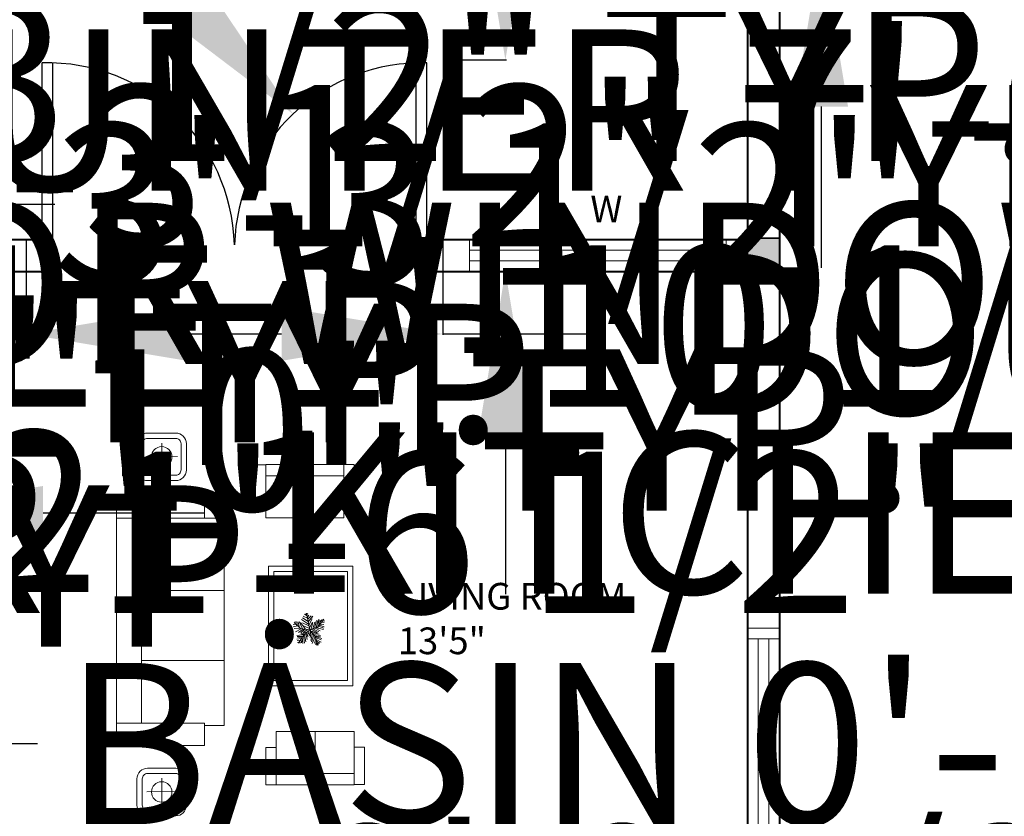
# Model space of a CAD drawing. Units: inches. Extents: x 7323 to 9737, y 2037 to 3322.
# Tile 14 of 19: x 9130 to 9314, y 2411 to 2560. Entities that reach past the tile are written whole.
import ezdxf

# ---------------------------------------------------------------- set-up
doc = ezdxf.new("R2010")
doc.units = ezdxf.units.IN
doc.header["$MEASUREMENT"] = 0
for name, color, linetype, lineweight in [('A-ANNO-DIMS', 2, 'Continuous', 18), ('A-ANNO-TEXT', 7, 'Continuous', 25), ('A-AREA-IDEN', 7, 'Continuous', 18), ('A-COLS', 1, 'Continuous', 35), ('A-DOOR', 4, 'Continuous', 25), ('A-FURN', 8, 'Continuous', 18), ('A-GLAZ', 4, 'Continuous', 18), ('A-WALL', 7, 'Continuous', 40)]:
    doc.layers.add(name, color=color, linetype=linetype, lineweight=lineweight)
doc.layers.add('A-COLS-PATT', color=18, linetype='Continuous', lineweight=13, true_color=0x000000)
doc.styles.get("Standard").update_dxf_attribs({"font": 'arial.ttf'})
doc.dimstyles.get("Standard").update_dxf_attribs({"dimtxt": 30.18, "dimasz": 30.18, "dimexe": 0.18, "dimexo": 0.0625, "dimgap": 0.09, "dimtad": 0, "dimtih": 1, "dimtoh": 1, "dimdec": 0, "dimzin": 0, "dimdsep": 46, "dimlunit": 3, "dimtxsty": 'Standard', "dimcen": 0.09, "dimadec": 0, "dimazin": 0, "dimtfac": 1, "dimtdec": 0, "dimtofl": 0, "dimtmove": 0, "dimatfit": 3, "dimfxl": 1, "dimtolj": 1, "dimtzin": 0, "dimarcsym": 0})

# ---------------------------------------------------------------- blocks, each defined once
blk = doc.blocks.new('*U4')
for p, q in [((-3.665, 19.273), (-27.574, 35.527)), ((-5.114, 28.097), (-24.676, 40.636)), ((-7.288, 39.707), (-21.778, 46.673)), ((-8.737, 47.138), (-17.069, 52.711)), ((-10.186, 53.64), (-13.084, 55.962)), ((0, 0), (-10.5, 57)), ((-9.099, 51.782), (-6.563, 55.962)), ((-7.65, 43.423), (-2.578, 49.46)), ((-5.839, 35.992), (4.667, 48.067)), ((-5.114, 27.632), (10.463, 46.673)), ((-2.941, 16.486), (8.652, 37.85)), ((27, 9), (48, 36)), ((27.127, 9.056), (31.112, 35.992)), ((38.719, 34.134), (41.979, 28.561)), ((44.153, 36.456), (45.239, 32.741)), ((-47.498, 19.737), (-55.83, 18.344)), ((-40.615, 13.7), (-55.105, 10.913)), ((-31.5, 4.5), (-52.5, 25.5)), ((-33.37, 6.269), (-52.207, 5.34)), ((-48.585, 21.131), (-49.309, 29.026)), ((-28.299, 3.483), (-47.86, -5.805)), ((-43.513, 28.561), (-42.427, 15.558)), ((-38.442, 26.239), (-34.819, 7.663)), ((-21.416, 3.018), (-38.079, -8.128)), ((-35.544, 28.097), (-24.314, 3.947)), ((0, 0), (-31.5, 4.5)), ((-14.533, 2.09), (-30.834, 25.31)), ((-15.982, 2.09), (-30.11, -9.521)), ((-24.314, 23.917), (-2.941, 13.7)), ((0, 0), (-22.5, -19.5)), ((-6.563, 1.161), (-21.416, -8.128)), ((-20.691, 13.7), (-1.129, 4.876)), ((-1.129, 6.734), (9.014, 26.704)), ((0, 0), (27, 9)), ((0, 0), (18, -22.5)), ((3.942, 1.625), (11.187, 24.381)), ((6.478, 1.625), (26.04, -8.592)), ((10.101, 3.483), (17.708, 26.239)), ((11.187, 3.483), (30.749, -5.805)), ((16.259, 5.805), (23.142, 31.348)), ((18.07, 5.805), (35.096, -3.483)), ((22.055, 7.198), (27.489, 32.277)), ((24.229, 7.663), (46.688, 1.625)), ((29.662, 12.307), (48.137, 6.269)), ((31.836, 30.883), (32.561, 16.486)), ((33.285, 16.486), (48.862, 10.913)), ((35.096, 32.741), (37.27, 22.524)), ((36.183, 19.737), (48.137, 17.88)), ((40.53, 25.775), (48.862, 24.846)), ((43.791, 29.954), (51.036, 30.883)), ((-17.431, -15.094), (-42.789, -18.809)), ((-28.299, -29.026), (-42.789, -31.348)), ((-24.314, -21.596), (-42.427, -22.06)), ((-26.849, -26.24), (-40.253, -25.775)), ((-22.5, -19.5), (-37.5, -45)), ((-15.257, -12.772), (-30.11, -12.772)), ((-29.023, -30.884), (-27.936, -43.887)), ((-25.038, -23.918), (-22.865, -45.281)), ((-20.691, -18.345), (-17.793, -44.352)), ((-6.563, -5.805), (-19.967, -9.985)), ((-17.069, -15.094), (-12.721, -40.172)), ((-13.446, -11.378), (-8.737, -32.741)), ((-9.461, -8.592), (-6.201, -23.453)), ((-4.752, -3.483), (-3.665, -14.629)), ((2.493, -3.019), (-1.491, -20.202)), ((1.769, -2.555), (24.229, -9.521)), ((5.029, -6.27), (2.131, -25.775)), ((9.014, -11.378), (3.58, -35.992)), ((14.085, -16.951), (6.478, -40.172)), ((7.565, -9.056), (32.198, -14.629)), ((18.07, -22.524), (8.289, -45.745)), ((12.274, -15.094), (36.907, -18.809)), ((20.244, -30.419), (15.897, -44.816)), ((16.259, -19.738), (36.183, -22.989)), ((18, -22.5), (27, -52.5)), ((18.433, -22.524), (40.53, -29.026)), ((19.157, -25.311), (38.719, -33.206)), ((21.331, -32.741), (39.081, -40.636)), ((-30.834, -34.135), (-42.427, -35.528)), ((-34.457, -39.708), (-40.978, -42.494)), ((-32.646, -36.921), (-31.921, -44.352)), ((22.78, -37.85), (19.519, -48.532)), ((22.78, -38.314), (34.372, -44.816)), ((24.591, -45.745), (23.142, -50.854)), ((24.591, -43.423), (30.749, -47.603)), ((26.764, -49.925), (28.213, -50.854))]:
    blk.add_line(p, q)
blk = doc.blocks.new('DOOR-PAIR-72')
for p, q in [((3, 6), (3, 39)), ((5, 3), (5, 39)), ((73, 3), (73, 39)), ((75, 6), (75, 39)), ((0, 6), (0, 0)), ((38.96, 6), (39.04, 6)), ((39, 6), (39, 5)), ((78, 6), (78, 0)), ((3, 3), (3, 0)), ((5, 3), (3, 3)), ((73, 3), (75, 3)), ((75, 3), (75, 0))]:
    blk.add_line(p, q)
for centre, start, end in [((4, 4), 1.6366, 91.6366), ((74, 4), 88.3634, 178.3634)]:
    blk.add_arc(centre, 35.01, start, end)
blk = doc.blocks.new('WIN-48')
for p, q in [((0, 0), (0, 6)), ((2, 0), (2, 6)), ((50, 0), (50, 6)), ((52, 0), (52, 6)), ((2, 4), (50, 4)), ((2, 2), (50, 2))]:
    blk.add_line(p, q)
blk = doc.blocks.new('WIN-48-SINGLE-JAMB')
for p, q in [((0, 6), (0, 0)), ((48, 6), (48, 0)), ((0, 4), (48, 4)), ((0, 2), (48, 2))]:
    blk.add_line(p, q)
blk = doc.blocks.new('COFFEE-TABLE')
for points in [[(15.8, 22.37), (15.8, 22.37), (0, 22.37), (0, 22.37), (0, 0), (0, 0), (15.8, 0), (15.8, 0)], [(14.8, 21.37), (1, 21.37), (1, 1), (14.8, 1)]]:
    blk.add_lwpolyline(points, close=True)
blk = doc.blocks.new('SOFA-THREE-SEAT')
for p, q in [((15.45, 29), (0, 29)), ((15.45, 29), (0, 29)), ((15.45, 15.91), (0, 15.91)), ((15.45, 15.91), (0, 15.91))]:
    blk.add_line(p, q)
for points in [[(20.12, 42.5), (20.12, 42.5), (3.63, 42.5), (3.63, 42.5), (3.63, 46.66), (3.63, 46.66), (20.12, 46.66), (20.12, 46.66)], [(20.12, 42.5), (20.12, 42.5), (3.63, 42.5), (3.63, 42.5), (3.63, 46.66), (3.63, 46.66), (20.12, 46.66), (20.12, 46.66)], [(15.45, 42.5), (15.45, 42.5), (20.12, 42.5), (20.12, 42.5), (20.12, 4.16), (20.12, 4.16), (15.45, 4.16), (15.45, 4.16)], [(15.45, 42.5), (15.45, 42.5), (20.12, 42.5), (20.12, 42.5), (20.12, 4.16), (20.12, 4.16), (15.45, 4.16), (15.45, 4.16)], [(20.12, 0), (20.12, 0), (3.63, 0), (3.63, 0), (3.63, 4.16), (3.63, 4.16), (20.12, 4.16), (20.12, 4.16)], [(20.12, 0), (20.12, 0), (3.63, 0), (3.63, 0), (3.63, 4.16), (3.63, 4.16), (20.12, 4.16), (20.12, 4.16)]]:
    blk.add_lwpolyline(points, close=True)
blk.add_lwpolyline([(15.45, 4.16), (15.45, 42.5), (15.45, 42.5), (0, 42.5), (0, 42.5), (0, 3.77), (0, 3.77), (3.63, 3.77)])
blk.add_lwpolyline([(15.45, 4.16), (15.45, 42.5), (15.45, 42.5), (0, 42.5), (0, 42.5), (0, 3.77), (0, 3.77), (3.63, 3.77)])
blk = doc.blocks.new('ARMCHAIR')
blk.add_line((9.19, 7.87), (9.19, 0))
for points in [[(0, 9.98), (0, 9.98), (1.9, 9.98), (1.9, 9.98), (1.9, 2.97), (1.9, 2.97), (0, 2.97), (0, 2.97)], [(16.51, 7.87), (16.51, 7.87), (1.9, 7.87), (1.9, 7.87), (1.9, 9.98), (1.9, 9.98), (16.51, 9.98), (16.51, 9.98)], [(16.51, 9.95), (16.51, 9.95), (18.41, 9.95), (18.41, 9.95), (18.41, 2.94), (18.41, 2.94), (16.51, 2.94), (16.51, 2.94)], [(16.51, 7.87), (16.51, 7.87), (1.88, 7.87), (1.88, 7.87), (1.88, 0), (1.88, 0), (16.51, 0), (16.51, 0)]]:
    blk.add_lwpolyline(points, close=True)
blk = doc.blocks.new('COL-PLAN-6IN')
blk.add_lwpolyline([(0, 6), (0, 6), (6.06, 6), (6.06, 6), (6.06, 0), (6.06, 0), (0, 0), (0, 0)], close=True)
blk = doc.blocks.new('*D37')
at = {"layer": 'A-ANNO-DIMS', "color": 0, "lineweight": -2, "transparency": 16777216}
for p, q in [((9279.75, 2656.48), (9279.75, 2686.66)), ((9272.01, 2626.3), (9279.93, 2626.3)), ((9272.01, 2574.3), (9279.93, 2574.3)), ((9279.75, 2544.12), (9279.75, 2513.94))]:
    blk.add_line(p, q, dxfattribs=at)
at = {"layer": 'A-ANNO-DIMS', "color": 0, "transparency": 16777216}
for points in [[(9274.72, 2656.48), (9284.78, 2656.48), (9279.75, 2626.3)], [(9274.72, 2544.12), (9284.78, 2544.12), (9279.75, 2574.3)]]:
    blk.add_solid(points, dxfattribs=at)
at = {"layer": 'Defpoints', "color": 0, "transparency": 16777216}
for p in [(9271.95, 2626.3), (9271.95, 2574.3), (9279.75, 2574.3)]:
    blk.add_point(p, dxfattribs=at)
at = {"layer": 'A-ANNO-DIMS', "color": 0, "transparency": 16777216, "insert": (9279.75, 2600.3), "char_height": 30.18, "attachment_point": 5}
blk.add_mtext('\\A1;WINDOW 4\'-4" TYP.', dxfattribs=at)
blk = doc.blocks.new('*D39')
at = {"layer": 'A-ANNO-DIMS', "color": 0, "lineweight": -2, "transparency": 16777216}
for p, q in [((8647.94, 2549.03), (8617.76, 2549.03)), ((8678.12, 2543.2), (8678.12, 2549.21)), ((8717.39, 2543.2), (8717.39, 2549.21)), ((8747.57, 2549.03), (8777.75, 2549.03))]:
    blk.add_line(p, q, dxfattribs=at)
at = {"layer": 'A-ANNO-DIMS', "color": 0, "transparency": 16777216}
for points in [[(8647.94, 2554.06), (8647.94, 2544), (8678.12, 2549.03)], [(8747.57, 2554.06), (8747.57, 2544), (8717.39, 2549.03)]]:
    blk.add_solid(points, dxfattribs=at)
at = {"layer": 'Defpoints', "color": 0, "transparency": 16777216}
for p in [(8717.39, 2549.03), (8678.12, 2543.14), (8717.39, 2543.14)]:
    blk.add_point(p, dxfattribs=at)
at = {"layer": 'A-ANNO-DIMS', "color": 0, "transparency": 16777216, "insert": (9057.19, 2549.03), "char_height": 30.18, "attachment_point": 5}
blk.add_mtext('\\A1;SINGLE DOOR 3\'-3 1/2" TYP.', dxfattribs=at)
blk = doc.blocks.new('*D41')
at = {"layer": 'A-ANNO-DIMS', "color": 0, "lineweight": -2, "transparency": 16777216}
for p, q in [((8661.59, 2428.04), (8661.59, 2458.22)), ((8661.59, 2458.22), (8691.77, 2458.22)), ((8657.46, 2397.86), (8661.77, 2397.86)), ((8657.46, 2369.86), (8661.77, 2369.86)), ((8661.59, 2339.68), (8661.59, 2309.5))]:
    blk.add_line(p, q, dxfattribs=at)
at = {"layer": 'A-ANNO-DIMS', "color": 0, "transparency": 16777216}
for points in [[(8656.56, 2428.04), (8666.62, 2428.04), (8661.59, 2397.86)], [(8656.56, 2339.68), (8666.62, 2339.68), (8661.59, 2369.86)]]:
    blk.add_solid(points, dxfattribs=at)
at = {"layer": 'Defpoints', "color": 0, "transparency": 16777216}
for p in [(8657.39, 2397.86), (8661.59, 2397.86), (8657.39, 2369.86)]:
    blk.add_point(p, dxfattribs=at)
at = {"layer": 'A-ANNO-DIMS', "color": 0, "transparency": 16777216, "insert": (8945.06, 2458.22), "char_height": 30.18, "attachment_point": 5}
blk.add_mtext('\\A1;VENT WINDOW 2\'-4" TYP.', dxfattribs=at)
blk = doc.blocks.new('*D43')
at = {"layer": 'A-ANNO-DIMS', "color": 0, "lineweight": -2, "transparency": 16777216}
for p, q in [((9108.94, 2438.75), (9108.94, 2468.93)), ((9104.01, 2408.57), (9109.12, 2408.57)), ((9104.01, 2375.3), (9109.12, 2375.3)), ((9108.94, 2345.12), (9108.94, 2314.94))]:
    blk.add_line(p, q, dxfattribs=at)
at = {"layer": 'A-ANNO-DIMS', "color": 0, "transparency": 16777216}
for points in [[(9103.91, 2438.75), (9113.97, 2438.75), (9108.94, 2408.57)], [(9103.91, 2345.12), (9113.97, 2345.12), (9108.94, 2375.3)]]:
    blk.add_solid(points, dxfattribs=at)
at = {"layer": 'Defpoints', "color": 0, "transparency": 16777216}
for p in [(9103.95, 2408.57), (9108.94, 2408.57), (9103.95, 2375.3)]:
    blk.add_point(p, dxfattribs=at)
at = {"layer": 'A-ANNO-DIMS', "color": 0, "transparency": 16777216, "insert": (9108.94, 2391.93), "char_height": 30.18, "attachment_point": 5}
blk.add_mtext('\\A1;BATH DOOR 2\'-9 1/2" TYP.', dxfattribs=at)
blk = doc.blocks.new('*D44')
at = {"layer": 'A-ANNO-DIMS', "color": 0, "lineweight": -2, "transparency": 16777216}
for p, q in [((9070.67, 2375.23), (9070.67, 2370.12)), ((9103.95, 2375.23), (9103.95, 2370.12)), ((9040.49, 2370.3), (9010.31, 2370.3)), ((9134.13, 2370.3), (9164.31, 2370.3))]:
    blk.add_line(p, q, dxfattribs=at)
at = {"layer": 'A-ANNO-DIMS', "color": 0, "transparency": 16777216}
for points in [[(9040.49, 2375.33), (9040.49, 2365.27), (9070.67, 2370.3)], [(9134.13, 2375.33), (9134.13, 2365.27), (9103.95, 2370.3)]]:
    blk.add_solid(points, dxfattribs=at)
at = {"layer": 'Defpoints', "color": 0, "transparency": 16777216}
for p in [(9070.67, 2375.3), (9103.95, 2375.3), (9103.95, 2370.3)]:
    blk.add_point(p, dxfattribs=at)
at = {"layer": 'A-ANNO-DIMS', "color": 0, "transparency": 16777216, "insert": (9291.8, 2370.3), "char_height": 30.18, "attachment_point": 5}
blk.add_mtext('\\A1;2\'-9 1/2" TYP.', dxfattribs=at)
blk = doc.blocks.new('*D47')
at = {"layer": 'A-ANNO-DIMS', "color": 0, "lineweight": -2, "transparency": 16777216}
for p, q in [((8809.55, 2464.49), (8779.37, 2464.49)), ((8839.73, 2461.79), (8839.73, 2464.67)), ((8858.14, 2461.79), (8858.14, 2464.67)), ((8888.32, 2464.49), (8918.5, 2464.49))]:
    blk.add_line(p, q, dxfattribs=at)
at = {"layer": 'A-ANNO-DIMS', "color": 0, "transparency": 16777216}
for points in [[(8809.55, 2469.52), (8809.55, 2459.46), (8839.73, 2464.49)], [(8888.32, 2469.52), (8888.32, 2459.46), (8858.14, 2464.49)]]:
    blk.add_solid(points, dxfattribs=at)
at = {"layer": 'Defpoints', "color": 0, "transparency": 16777216}
for p in [(8858.14, 2464.49), (8839.73, 2461.73), (8858.14, 2461.73)]:
    blk.add_point(p, dxfattribs=at)
at = {"layer": 'A-ANNO-DIMS', "color": 0, "transparency": 16777216, "insert": (9164.9, 2464.49), "char_height": 30.18, "attachment_point": 5}
blk.add_mtext('\\A1;ARMCHAIR 1\'-6 1/2" TYP.', dxfattribs=at)
blk = doc.blocks.new('*D51')
at = {"layer": 'A-ANNO-DIMS', "color": 0, "lineweight": -2, "transparency": 16777216}
for p, q in [((9130.95, 2513.23), (9130.95, 2501.42)), ((9208.95, 2513.23), (9208.95, 2501.42)), ((9161.13, 2501.6), (9178.77, 2501.6)), ((9208.95, 2501.6), (9239.13, 2501.6))]:
    blk.add_line(p, q, dxfattribs=at)
at = {"layer": 'A-ANNO-DIMS', "color": 0, "transparency": 16777216}
for points in [[(9161.13, 2506.63), (9161.13, 2496.57), (9130.95, 2501.6)], [(9178.77, 2506.63), (9178.77, 2496.57), (9208.95, 2501.6)]]:
    blk.add_solid(points, dxfattribs=at)
at = {"layer": 'Defpoints', "color": 0, "transparency": 16777216}
for p in [(9130.95, 2513.3), (9208.95, 2513.3), (9208.95, 2501.6)]:
    blk.add_point(p, dxfattribs=at)
at = {"layer": 'A-ANNO-DIMS', "color": 0, "transparency": 16777216, "insert": (9492.09, 2501.6), "char_height": 30.18, "attachment_point": 5}
blk.add_mtext('\\A1;DOUBLE DOOR 6\'-6" TYP.', dxfattribs=at)
blk = doc.blocks.new('*D52')
at = {"layer": 'A-ANNO-DIMS', "color": 0, "lineweight": -2, "transparency": 16777216}
for p, q in [((9220.65, 2583.03), (9220.65, 2613.21)), ((9209.01, 2552.85), (9220.83, 2552.85)), ((9209.01, 2513.3), (9220.83, 2513.3)), ((9220.65, 2483.12), (9220.65, 2452.94))]:
    blk.add_line(p, q, dxfattribs=at)
at = {"layer": 'A-ANNO-DIMS', "color": 0, "transparency": 16777216}
for points in [[(9215.62, 2583.03), (9225.68, 2583.03), (9220.65, 2552.85)], [(9215.62, 2483.12), (9225.68, 2483.12), (9220.65, 2513.3)]]:
    blk.add_solid(points, dxfattribs=at)
at = {"layer": 'Defpoints', "color": 0, "transparency": 16777216}
for p in [(9208.95, 2552.85), (9220.65, 2552.85), (9208.95, 2513.3)]:
    blk.add_point(p, dxfattribs=at)
at = {"layer": 'A-ANNO-DIMS', "color": 0, "transparency": 16777216, "insert": (9220.65, 2533.07), "char_height": 30.18, "attachment_point": 5}
blk.add_mtext('\\A1;3\'-3 1/2" TYP.', dxfattribs=at)
blk = doc.blocks.new('*D53')
at = {"layer": 'A-ANNO-DIMS', "color": 0, "lineweight": -2, "transparency": 16777216}
for p, q in [((8826.85, 2511.06), (8796.67, 2511.06)), ((8857.03, 2503.93), (8857.03, 2511.24)), ((8905.03, 2503.93), (8905.03, 2511.24)), ((8935.21, 2511.06), (8965.39, 2511.06))]:
    blk.add_line(p, q, dxfattribs=at)
at = {"layer": 'A-ANNO-DIMS', "color": 0, "transparency": 16777216}
for points in [[(8826.85, 2516.09), (8826.85, 2506.03), (8857.03, 2511.06)], [(8935.21, 2516.09), (8935.21, 2506.03), (8905.03, 2511.06)]]:
    blk.add_solid(points, dxfattribs=at)
at = {"layer": 'Defpoints', "color": 0, "transparency": 16777216}
for p in [(8905.03, 2511.06), (8857.03, 2503.86), (8905.03, 2503.86)]:
    blk.add_point(p, dxfattribs=at)
at = {"layer": 'A-ANNO-DIMS', "color": 0, "transparency": 16777216, "insert": (9261.3, 2511.06), "char_height": 30.18, "attachment_point": 5}
blk.add_mtext('\\A1;INTERIOR WINDOW 4\'-0" TYP.', dxfattribs=at)
blk = doc.blocks.new('*D59')
at = {"layer": 'A-ANNO-DIMS', "color": 0, "lineweight": -2, "transparency": 16777216}
for p, q in [((9064.67, 2473.96), (9064.67, 2467.95)), ((9103.95, 2473.96), (9103.95, 2467.95)), ((9034.49, 2468.13), (9004.31, 2468.13)), ((9134.13, 2468.13), (9164.31, 2468.13))]:
    blk.add_line(p, q, dxfattribs=at)
at = {"layer": 'A-ANNO-DIMS', "color": 0, "transparency": 16777216}
for points in [[(9034.49, 2473.16), (9034.49, 2463.1), (9064.67, 2468.13)], [(9134.13, 2473.16), (9134.13, 2463.1), (9103.95, 2468.13)]]:
    blk.add_solid(points, dxfattribs=at)
at = {"layer": 'Defpoints', "color": 0, "transparency": 16777216}
for p in [(9064.67, 2474.02), (9103.95, 2474.02), (9103.95, 2468.13)]:
    blk.add_point(p, dxfattribs=at)
at = {"layer": 'A-ANNO-DIMS', "color": 0, "transparency": 16777216, "insert": (9458.35, 2468.13), "char_height": 30.18, "attachment_point": 5}
blk.add_mtext('\\A1;KITCHEN DOOR 3\'-3 1/2" TYP.', dxfattribs=at)
blk = doc.blocks.new('*D60')
at = {"layer": 'A-ANNO-DIMS', "color": 0, "lineweight": -2, "transparency": 16777216}
for p, q in [((9109.84, 2540.48), (9109.84, 2570.66)), ((9104.01, 2510.3), (9110.02, 2510.3)), ((9104.01, 2474.02), (9110.02, 2474.02)), ((9109.84, 2443.84), (9109.84, 2413.66))]:
    blk.add_line(p, q, dxfattribs=at)
at = {"layer": 'A-ANNO-DIMS', "color": 0, "transparency": 16777216}
for points in [[(9104.81, 2540.48), (9114.87, 2540.48), (9109.84, 2510.3)], [(9104.81, 2443.84), (9114.87, 2443.84), (9109.84, 2474.02)]]:
    blk.add_solid(points, dxfattribs=at)
at = {"layer": 'Defpoints', "color": 0, "transparency": 16777216}
for p in [(9103.95, 2510.3), (9109.84, 2510.3), (9103.95, 2474.02)]:
    blk.add_point(p, dxfattribs=at)
at = {"layer": 'A-ANNO-DIMS', "color": 0, "transparency": 16777216, "insert": (9109.84, 2492.16), "char_height": 30.18, "attachment_point": 5}
blk.add_mtext('\\A1;3\'-0 1/2" TYP.', dxfattribs=at)
blk = doc.blocks.new('*D62')
at = {"layer": 'A-ANNO-DIMS', "color": 0, "lineweight": -2, "transparency": 16777216}
for p, q in [((9134.53, 2605.32), (9134.53, 2593.82)), ((9201.18, 2605.32), (9201.18, 2593.82)), ((9164.71, 2594), (9171, 2594)), ((9201.18, 2594), (9231.36, 2594))]:
    blk.add_line(p, q, dxfattribs=at)
at = {"layer": 'A-ANNO-DIMS', "color": 0, "transparency": 16777216}
for points in [[(9164.71, 2599.03), (9164.71, 2588.97), (9134.53, 2594)], [(9171, 2599.03), (9171, 2588.97), (9201.18, 2594)]]:
    blk.add_solid(points, dxfattribs=at)
at = {"layer": 'Defpoints', "color": 0, "transparency": 16777216}
for p in [(9134.53, 2605.38), (9201.18, 2605.38), (9201.18, 2594)]:
    blk.add_point(p, dxfattribs=at)
at = {"layer": 'A-ANNO-DIMS', "color": 0, "transparency": 16777216, "insert": (9358.59, 2594), "char_height": 30.18, "attachment_point": 5}
blk.add_mtext('\\A1;5\'-6 1/2" TYP.', dxfattribs=at)
blk = doc.blocks.new('*D63')
at = {"layer": 'A-ANNO-DIMS', "color": 0, "lineweight": -2, "transparency": 16777216}
for p, q in [((8744.72, 2466.22), (8744.72, 2496.4)), ((8744.72, 2496.4), (8774.9, 2496.4)), ((8741.46, 2436.04), (8744.9, 2436.04)), ((8741.46, 2413.86), (8744.9, 2413.86)), ((8744.72, 2383.68), (8744.72, 2353.5))]:
    blk.add_line(p, q, dxfattribs=at)
at = {"layer": 'A-ANNO-DIMS', "color": 0, "transparency": 16777216}
for points in [[(8739.69, 2466.22), (8749.75, 2466.22), (8744.72, 2436.04)], [(8739.69, 2383.68), (8749.75, 2383.68), (8744.72, 2413.86)]]:
    blk.add_solid(points, dxfattribs=at)
at = {"layer": 'Defpoints', "color": 0, "transparency": 16777216}
for p in [(8741.39, 2436.04), (8744.72, 2436.04), (8741.39, 2413.86)]:
    blk.add_point(p, dxfattribs=at)
at = {"layer": 'A-ANNO-DIMS', "color": 0, "transparency": 16777216, "insert": (9003.76, 2496.4), "char_height": 30.18, "attachment_point": 5}
blk.add_mtext('\\A1;APPLIANCE 1\'-10" TYP.', dxfattribs=at)
blk = doc.blocks.new('*D65')
at = {"layer": 'A-ANNO-DIMS', "color": 0, "lineweight": -2, "transparency": 16777216}
for p, q in [((9024.02, 2513.3), (9024.02, 2543.48)), ((9024.02, 2543.48), (9054.2, 2543.48)), ((9036.56, 2513.3), (9023.84, 2513.3)), ((9024.02, 2459.48), (9024.02, 2483.12)), ((9036.56, 2429.3), (9023.84, 2429.3))]:
    blk.add_line(p, q, dxfattribs=at)
at = {"layer": 'A-ANNO-DIMS', "color": 0, "transparency": 16777216}
for points in [[(9018.99, 2483.12), (9029.05, 2483.12), (9024.02, 2513.3)], [(9018.99, 2459.48), (9029.05, 2459.48), (9024.02, 2429.3)]]:
    blk.add_solid(points, dxfattribs=at)
at = {"layer": 'Defpoints', "color": 0, "transparency": 16777216}
for p in [(9024.02, 2513.3), (9036.62, 2513.3), (9036.62, 2429.3)]:
    blk.add_point(p, dxfattribs=at)
at = {"layer": 'A-ANNO-DIMS', "color": 0, "transparency": 16777216, "insert": (9256.18, 2543.48), "char_height": 30.18, "attachment_point": 5}
blk.add_mtext('\\A1;COUNTER 7\'-0" TYP.', dxfattribs=at)
blk = doc.blocks.new('*D66')
at = {"layer": 'A-ANNO-DIMS', "color": 0, "lineweight": -2, "transparency": 16777216}
for p, q in [((9006.44, 2525.9), (8976.26, 2525.9)), ((9036.62, 2513.36), (9036.62, 2526.08)), ((9075.95, 2513.36), (9075.95, 2526.08)), ((9106.13, 2525.9), (9136.31, 2525.9))]:
    blk.add_line(p, q, dxfattribs=at)
at = {"layer": 'A-ANNO-DIMS', "color": 0, "transparency": 16777216}
for points in [[(9006.44, 2530.93), (9006.44, 2520.87), (9036.62, 2525.9)], [(9106.13, 2530.93), (9106.13, 2520.87), (9075.95, 2525.9)]]:
    blk.add_solid(points, dxfattribs=at)
at = {"layer": 'Defpoints', "color": 0, "transparency": 16777216}
for p in [(9075.95, 2525.9), (9036.62, 2513.3), (9075.95, 2513.3)]:
    blk.add_point(p, dxfattribs=at)
at = {"layer": 'A-ANNO-DIMS', "color": 0, "transparency": 16777216, "insert": (9263.53, 2525.9), "char_height": 30.18, "attachment_point": 5}
blk.add_mtext('\\A1;3\'-3 1/2" TYP.', dxfattribs=at)
blk = doc.blocks.new('*D69')
at = {"layer": 'A-ANNO-DIMS', "color": 0, "lineweight": -2, "transparency": 16777216}
for p, q in [((8836.58, 2472.89), (8836.58, 2503.07)), ((8836.58, 2503.07), (8866.76, 2503.07)), ((8839.88, 2442.71), (8836.4, 2442.71)), ((8839.88, 2420.33), (8836.4, 2420.33)), ((8836.58, 2390.15), (8836.58, 2359.97))]:
    blk.add_line(p, q, dxfattribs=at)
at = {"layer": 'A-ANNO-DIMS', "color": 0, "transparency": 16777216}
for points in [[(8831.55, 2472.89), (8841.61, 2472.89), (8836.58, 2442.71)], [(8831.55, 2390.15), (8841.61, 2390.15), (8836.58, 2420.33)]]:
    blk.add_solid(points, dxfattribs=at)
at = {"layer": 'Defpoints', "color": 0, "transparency": 16777216}
for p in [(8836.58, 2442.71), (8839.94, 2442.71), (8839.94, 2420.33)]:
    blk.add_point(p, dxfattribs=at)
at = {"layer": 'A-ANNO-DIMS', "color": 0, "transparency": 16777216, "insert": (9169.54, 2503.07), "char_height": 30.18, "attachment_point": 5}
blk.add_mtext('\\A1;COFFEE TABLE 1\'-10 1/2" TYP.', dxfattribs=at)
blk = doc.blocks.new('*D73')
at = {"layer": 'A-ANNO-DIMS', "color": 0, "lineweight": -2, "transparency": 16777216}
for p, q in [((9061.59, 2423.36), (9061.59, 2425.15)), ((9072.75, 2423.36), (9072.75, 2425.15)), ((9031.41, 2424.97), (9001.23, 2424.97)), ((9102.93, 2424.97), (9133.11, 2424.97))]:
    blk.add_line(p, q, dxfattribs=at)
at = {"layer": 'A-ANNO-DIMS', "color": 0, "transparency": 16777216}
for points in [[(9031.41, 2430), (9031.41, 2419.94), (9061.59, 2424.97)], [(9102.93, 2430), (9102.93, 2419.94), (9072.75, 2424.97)]]:
    blk.add_solid(points, dxfattribs=at)
at = {"layer": 'Defpoints', "color": 0, "transparency": 16777216}
for p in [(9061.59, 2423.3), (9072.75, 2424.97), (9072.75, 2423.3)]:
    blk.add_point(p, dxfattribs=at)
at = {"layer": 'A-ANNO-DIMS', "color": 0, "transparency": 16777216, "insert": (9305.36, 2424.97), "char_height": 30.18, "attachment_point": 5}
blk.add_mtext('\\A1;BASIN 0\'-11" TYP.', dxfattribs=at)
blk = doc.blocks.new('*D74')
at = {"layer": 'A-ANNO-DIMS', "color": 0, "lineweight": -2, "transparency": 16777216}
for p, q in [((9059.91, 2453.48), (9059.91, 2483.66)), ((9059.91, 2483.66), (9090.09, 2483.66)), ((9061.53, 2423.3), (9059.73, 2423.3)), ((9061.53, 2413.24), (9059.73, 2413.24)), ((9059.91, 2383.06), (9059.91, 2352.88))]:
    blk.add_line(p, q, dxfattribs=at)
at = {"layer": 'A-ANNO-DIMS', "color": 0, "transparency": 16777216}
for points in [[(9054.88, 2453.48), (9064.94, 2453.48), (9059.91, 2423.3)], [(9054.88, 2383.06), (9064.94, 2383.06), (9059.91, 2413.24)]]:
    blk.add_solid(points, dxfattribs=at)
at = {"layer": 'Defpoints', "color": 0, "transparency": 16777216}
for p in [(9059.91, 2423.3), (9061.59, 2423.3), (9061.59, 2413.24)]:
    blk.add_point(p, dxfattribs=at)
at = {"layer": 'A-ANNO-DIMS', "color": 0, "transparency": 16777216, "insert": (9193.89, 2483.66), "char_height": 30.18, "attachment_point": 5}
blk.add_mtext('\\A1;0\'-10" TYP.', dxfattribs=at)
blk = doc.blocks.new('*D79')
at = {"layer": 'A-ANNO-DIMS', "color": 0, "lineweight": -2, "transparency": 16777216}
for p, q in [((8871.1, 2395.97), (8871.1, 2394.46)), ((8880.36, 2395.97), (8880.36, 2394.46)), ((8840.92, 2394.64), (8810.74, 2394.64)), ((8910.54, 2394.64), (8940.72, 2394.64))]:
    blk.add_line(p, q, dxfattribs=at)
at = {"layer": 'A-ANNO-DIMS', "color": 0, "transparency": 16777216}
for points in [[(8840.92, 2399.67), (8840.92, 2389.61), (8871.1, 2394.64)], [(8910.54, 2399.67), (8910.54, 2389.61), (8880.36, 2394.64)]]:
    blk.add_solid(points, dxfattribs=at)
at = {"layer": 'Defpoints', "color": 0, "transparency": 16777216}
for p in [(8871.1, 2396.03), (8880.36, 2396.03), (8880.36, 2394.64)]:
    blk.add_point(p, dxfattribs=at)
at = {"layer": 'A-ANNO-DIMS', "color": 0, "transparency": 16777216, "insert": (9195.57, 2394.64), "char_height": 30.18, "attachment_point": 5}
blk.add_mtext('\\A1;SIDE TABLE 0\'-9 1/2" TYP.', dxfattribs=at)
blk = doc.blocks.new('*D111')
at = {"layer": 'A-ANNO-DIMS', "color": 0, "lineweight": -2, "transparency": 16777216}
for p, q in [((9011.299226, 2468.388949), (8981.119226, 2468.388949)), ((9041.479226, 2433.251449), (9041.479226, 2468.568949)), ((9066.478924, 2433.251449), (9066.478924, 2468.568949)), ((9096.658924, 2468.388949), (9126.838924, 2468.388949))]:
    blk.add_line(p, q, dxfattribs=at)
at = {"layer": 'A-ANNO-DIMS', "color": 0, "transparency": 16777216}
for points in [[(9011.299226, 2473.418949), (9011.299226, 2463.358949), (9041.479226, 2468.388949)], [(9096.658924, 2473.418949), (9096.658924, 2463.358949), (9066.478924, 2468.388949)]]:
    blk.add_solid(points, dxfattribs=at)
at = {"layer": 'Defpoints', "color": 0, "transparency": 16777216}
for p in [(9066.478924, 2468.388949), (9041.479226, 2433.188949), (9066.478924, 2433.188949)]:
    blk.add_point(p, dxfattribs=at)
at = {"layer": 'A-ANNO-DIMS', "color": 0, "transparency": 16777216, "insert": (9167.299306, 2468.388949), "char_height": 30.18, "attachment_point": 5}
blk.add_mtext('\\A1;2\'-1"', dxfattribs=at)
blk = doc.blocks.new('*D126')
at = {"layer": 'A-ANNO-DIMS', "color": 0, "lineweight": -2, "transparency": 16777216}
for p, q in [((9109.28, 2586.63), (9139.46, 2586.63)), ((9139.46, 2586.63), (9160.18, 2564.69)), ((9204.86, 2517.3), (9205.04, 2517.3)), ((9204.95, 2517.21), (9204.95, 2517.39))]:
    blk.add_line(p, q, dxfattribs=at)
at = {"layer": 'A-ANNO-DIMS', "color": 0, "transparency": 16777216}
blk.add_solid([(9163.84, 2568.15), (9156.52, 2561.24), (9180.9, 2542.75)], dxfattribs=at)
at = {"layer": 'Defpoints', "color": 0, "transparency": 16777216}
for p in [(9180.9, 2542.75), (9204.95, 2517.3)]:
    blk.add_point(p, dxfattribs=at)
at = {"layer": 'A-ANNO-DIMS', "color": 0, "transparency": 16777216, "insert": (9009.88, 2586.63), "char_height": 30.18, "attachment_point": 5}
blk.add_mtext('\\A1;4X R2\'-11"', dxfattribs=at)

msp = doc.modelspace()

# ---------------------------------------------------------------- hatches: boundary and pattern name
at = {"layer": 'A-COLS-PATT'}
h = msp.add_hatch(color=256, dxfattribs=at)
h.dxf.hatch_style = 1
h.paths.add_polyline_path([(8915.39, 2189.86), (8908.77, 2189.86), (8908.77, 2183.86), (8915.39, 2183.86)])
h.paths.add_polyline_path([(8657.61, 2189.86), (8651.55, 2189.86), (8651.55, 2183.86), (8657.61, 2183.86)])
h.paths.add_polyline_path([(8814.13, 2189.86), (8807.39, 2189.86), (8807.39, 2183.86), (8814.13, 2183.86)])
h.paths.add_polyline_path([(8813.39, 2317.86), (8807.36, 2317.86), (8807.36, 2311.86), (8813.39, 2311.86)])
h.paths.add_polyline_path([(8915.34, 2313.13), (8909.39, 2313.13), (8909.39, 2307.13), (8915.34, 2307.13)])
h.paths.add_polyline_path([(8657.62, 2317.86), (8657.39, 2317.86), (8657.39, 2318.08), (8651.55, 2318.08), (8651.55, 2312.08), (8657.62, 2312.08)])
h.paths.add_polyline_path([(8915.39, 2671.84), (8909.37, 2671.84), (8909.37, 2665.86), (8909.39, 2665.86), (8915.39, 2665.84)])
h.paths.add_polyline_path([(8657.59, 2671.81), (8651.52, 2671.81), (8651.52, 2665.81), (8657.39, 2665.81), (8657.39, 2665.86)])
h.paths.add_polyline_path([(8915.28, 2503.94), (8909.39, 2503.94), (8909.39, 2503.86), (8909.22, 2497.94), (8915.28, 2497.94)])
h.paths.add_polyline_path([(8657.53, 2503.86), (8657.39, 2503.86), (8651.46, 2503.96), (8651.46, 2497.96), (8657.53, 2497.96)])
h.paths.add_polyline_path([(9014.24, 2519.3), (9013.95, 2519.3), (9008.18, 2519.31), (9008.18, 2513.31), (9014.24, 2513.31)])
h.paths.add_polyline_path([(9013.95, 2687.3), (9007.95, 2687.3), (9007.95, 2681.3), (9013.95, 2681.3)])
h.paths.add_polyline_path([(9271.95, 2687.3), (9266.01, 2687.3), (9266.01, 2681.35), (9271.95, 2681.35)])
h.paths.add_polyline_path([(9271.95, 2205.3), (9265.32, 2205.3), (9265.32, 2199.3), (9271.95, 2199.3)])
h.paths.add_polyline_path([(9170.68, 2205.3), (9163.95, 2205.3), (9163.95, 2199.3), (9170.68, 2199.3)])
h.paths.add_polyline_path([(9013.95, 2205.3), (9007.95, 2205.3), (9007.95, 2199.3), (9013.95, 2199.3)])
h.paths.add_polyline_path([(9271.95, 2519.51), (9265.95, 2519.51), (9265.95, 2519.3), (9265.93, 2513.51), (9271.95, 2513.51)])
h.paths.add_polyline_path([(9271.95, 2328.64), (9265.95, 2328.64), (9265.95, 2322.64), (9271.95, 2322.64)])
h.paths.add_polyline_path([(9014.35, 2333.3), (9013.95, 2333.3), (9013.95, 2333.58), (9008.29, 2333.58), (9008.29, 2327.58), (9014.35, 2327.58)])

# ---------------------------------------------------------------- linework, layer by layer
at = {"layer": 'A-FURN'}
for p, q in [((9156.37, 2481.2), (9156.37, 2475.82)), ((9153.53, 2478.61), (9159.27, 2478.69)), ((9156.37, 2418.5), (9156.37, 2413.12)), ((9153.53, 2415.92), (9159.27, 2415.99))]:
    msp.add_line(p, q, dxfattribs=at)
for points in [[(9151.69, 2481.07, -0.414214), (9153.69, 2483.07), (9158.94, 2483.07, -0.414214), (9160.94, 2481.07), (9160.94, 2476.16, -0.414214), (9158.94, 2474.16), (9153.69, 2474.16, -0.414214), (9151.69, 2476.16)], [(9152.69, 2481.07, -0.414214), (9153.69, 2482.07), (9158.94, 2482.07, -0.414214), (9159.94, 2481.07), (9159.94, 2476.16, -0.414214), (9158.94, 2475.16), (9153.69, 2475.16, -0.414214), (9152.69, 2476.16)], [(9151.69, 2418.37, -0.414214), (9153.69, 2420.37), (9158.94, 2420.37, -0.414214), (9160.94, 2418.37), (9160.94, 2413.46, -0.414214), (9158.94, 2411.46), (9153.69, 2411.46, -0.414214), (9151.69, 2413.46)], [(9152.69, 2418.37, -0.414214), (9153.69, 2419.37), (9158.94, 2419.37, -0.414214), (9159.94, 2418.37), (9159.94, 2413.46, -0.414214), (9158.94, 2412.46), (9153.69, 2412.46, -0.414214), (9152.69, 2413.46)]]:
    msp.add_lwpolyline(points, format="xyb", close=True, dxfattribs=at)
for centre in [(9156.32, 2478.61), (9156.32, 2415.92)]:
    msp.add_circle(centre, 1.91, dxfattribs=at)
at = {"layer": 'A-WALL'}
for p, q in [((9271.95, 2687.3), (9271.95, 2199.3)), ((9265.95, 2681.3), (9265.95, 2519.3)), ((9073.95, 2519.3), (9135.95, 2519.3)), ((9203.95, 2519.3), (9265.95, 2519.3)), ((9013.95, 2513.3), (9133.95, 2513.3)), ((9205.95, 2513.3), (9265.95, 2513.3)), ((9265.95, 2513.3), (9265.95, 2205.3))]:
    msp.add_line(p, q, dxfattribs=at)

# ---------------------------------------------------------------- block references
at = {"layer": 'A-COLS'}
msp.add_blockref('COL-PLAN-6IN', (9265.93, 2513.51), dxfattribs=at)
at = {"layer": 'A-DOOR'}
msp.add_blockref('DOOR-PAIR-72', (9130.95, 2513.3), dxfattribs=at)
at = {"layer": 'A-FURN', "extrusion": (0, 0, -1), "zscale": -1}
for name, p in [('ARMCHAIR', (-9192.32, 2467.18)), ('SOFA-THREE-SEAT', (-9167.99, 2424.61)), ('COFFEE-TABLE', (-9192.11, 2435.77))]:
    msp.add_blockref(name, p, dxfattribs=at)
at = {"layer": 'A-FURN', "xscale": 0.0555195490297955, "yscale": 0.0555195490297955, "zscale": 0.0555195490297955}
msp.add_blockref('*U4', (9184.02, 2446.23), dxfattribs=at)
at = {"layer": 'A-FURN', "extrusion": (0, 0, -1), "zscale": -1, "rotation": 180}
msp.add_blockref('ARMCHAIR', (-9175.84, 2427.24), dxfattribs=at)
at = {"layer": 'A-GLAZ'}
for name, p, rotation in [('WIN-48-SINGLE-JAMB', (9261.95, 2519.3), 180), ('WIN-48', (9265.95, 2446.56), 270.000000000004)]:
    msp.add_blockref(name, p, dxfattribs=dict(at, rotation=rotation))

# ---------------------------------------------------------------- texts
at = {"layer": 'A-ANNO-TEXT', "insert": (9236.55, 2527.46), "char_height": 5, "attachment_point": 1}
msp.add_mtext_dynamic_manual_height_columns('W', width=26.304, gutter_width=1, heights=[0], dxfattribs=at)
at = {"layer": 'A-AREA-IDEN', "insert": (9200.51, 2455.03), "char_height": 5, "attachment_point": 1}
msp.add_mtext_dynamic_manual_height_columns('LIVING ROOM\\P13\'5"', width=54.2256, gutter_width=1, heights=[0], dxfattribs=at)

# ---------------------------------------------------------------- dimensions: what is measured, and where the dimension line sits
at = {"layer": 'A-ANNO-DIMS'}
for base, p1, p2, angle, text, picture, middle in [((9279.75, 2574.3), (9271.95, 2626.3), (9271.95, 2574.3), 270, 'WINDOW <> TYP.', '*D37', (9279.75, 2600.3)), ((8836.58, 2442.71), (8839.94, 2420.33), (8839.94, 2442.71), 90, 'COFFEE TABLE <> TYP.', '*D69', (9169.54, 2503.07)), ((9024.02, 2513.3), (9036.62, 2429.3), (9036.62, 2513.3), 90, 'COUNTER <> TYP.', '*D65', (9256.18, 2543.48)), ((9220.6454, 2552.8475), (9208.9454, 2513.2952), (9208.9454, 2552.8475), 90, '<> TYP.', '*D52', (9220.6454, 2533.0713)), ((9109.84, 2510.3), (9103.95, 2474.02), (9103.95, 2510.3), 90, '<> TYP.', '*D60', (9109.84, 2492.16)), ((8744.72, 2436.04), (8741.39, 2413.86), (8741.39, 2436.04), 90, 'APPLIANCE <> TYP.', '*D63', (9003.76, 2496.4)), ((8661.59, 2397.86), (8657.39, 2369.86), (8657.39, 2397.86), 90, 'VENT WINDOW <> TYP.', '*D41', (8945.06, 2458.22)), ((9059.91, 2423.3), (9061.59, 2413.24), (9061.59, 2423.3), 90, '<> TYP.', '*D74', (9193.89, 2483.66)), ((9108.94, 2408.57), (9103.95, 2375.3), (9103.95, 2408.57), 90, 'BATH DOOR <> TYP.', '*D43', (9108.94, 2391.93))]:
    dim = msp.add_linear_dim(base=base, p1=p1, p2=p2, angle=angle, text=text, dimstyle='Standard', override={"dimdec": 1, "dimlfac": 1, "dimrnd": 0, "dimzin": 1, "dimdsep": 46, "dimlunit": 4, "dimfrac": 2}, dxfattribs=at)
    dim.commit()
    dim.dimension.update_dxf_attribs({"geometry": picture, "text_midpoint": middle})
for base, p1, p2, text, picture, middle in [((8717.39, 2549.03), (8678.12, 2543.14), (8717.39, 2543.14), 'SINGLE DOOR <> TYP.', '*D39', (9057.19, 2549.03)), ((9201.1793, 2593.9956), (9134.5282, 2605.3825), (9201.1793, 2605.3825), '<> TYP.', '*D62', (9358.5924, 2593.9956)), ((8905.03, 2511.06), (8857.03, 2503.86), (8905.03, 2503.86), 'INTERIOR WINDOW <> TYP.', '*D53', (9261.3, 2511.06)), ((9208.95, 2501.6), (9130.95, 2513.3), (9208.95, 2513.3), 'DOUBLE DOOR <> TYP.', '*D51', (9492.09, 2501.6)), ((9075.95, 2525.9), (9036.62, 2513.3), (9075.95, 2513.3), '<> TYP.', '*D66', (9263.53, 2525.9)), ((9103.95, 2468.13), (9064.67, 2474.02), (9103.95, 2474.02), 'KITCHEN DOOR <> TYP.', '*D59', (9458.35, 2468.13)), ((8858.14, 2464.49), (8839.73, 2461.73), (8858.14, 2461.73), 'ARMCHAIR <> TYP.', '*D47', (9164.9, 2464.49)), ((8880.36, 2394.64), (8871.1, 2396.03), (8880.36, 2396.03), 'SIDE TABLE <> TYP.', '*D79', (9195.57, 2394.64)), ((9072.75, 2424.97), (9061.59, 2423.3), (9072.75, 2423.3), 'BASIN <> TYP.', '*D73', (9305.36, 2424.97)), ((9103.95, 2370.3), (9070.67, 2375.3), (9103.95, 2375.3), '<> TYP.', '*D44', (9291.8, 2370.3))]:
    dim = msp.add_linear_dim(base=base, p1=p1, p2=p2, text=text, dimstyle='Standard', override={"dimdec": 1, "dimlfac": 1, "dimrnd": 0, "dimzin": 1, "dimdsep": 46, "dimlunit": 4, "dimfrac": 2}, dxfattribs=at)
    dim.commit()
    dim.dimension.update_dxf_attribs({"geometry": picture, "text_midpoint": middle})
dim = msp.add_radius_dim(center=(9204.95, 2517.3), mpoint=(9180.9, 2542.75), text='4X <>', dimstyle='Standard', override={"dimdec": 1, "dimlfac": 1, "dimrnd": 0, "dimzin": 1, "dimdsep": 46, "dimlunit": 4, "dimfrac": 2}, dxfattribs=at)
dim.commit()
dim.dimension.update_dxf_attribs({"geometry": '*D126', "text_midpoint": (9009.88, 2586.63)})
dim = msp.add_linear_dim(base=(9066.48, 2468.39), p1=(9041.48, 2433.19), p2=(9066.48, 2433.19), dimstyle='Standard', override={"dimdec": 1, "dimlfac": 1, "dimrnd": 0, "dimzin": 1, "dimdsep": 46, "dimlunit": 4, "dimfrac": 2}, dxfattribs=at)
dim.commit()
dim.dimension.update_dxf_attribs({"geometry": '*D111', "text_midpoint": (9167.3, 2468.39)})

doc.saveas('drawing.dxf')
